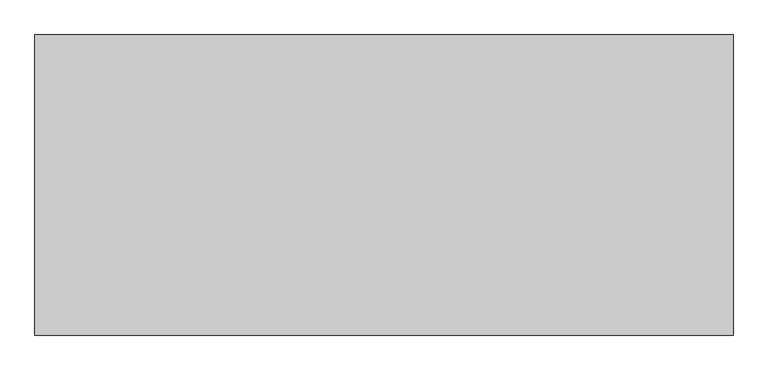
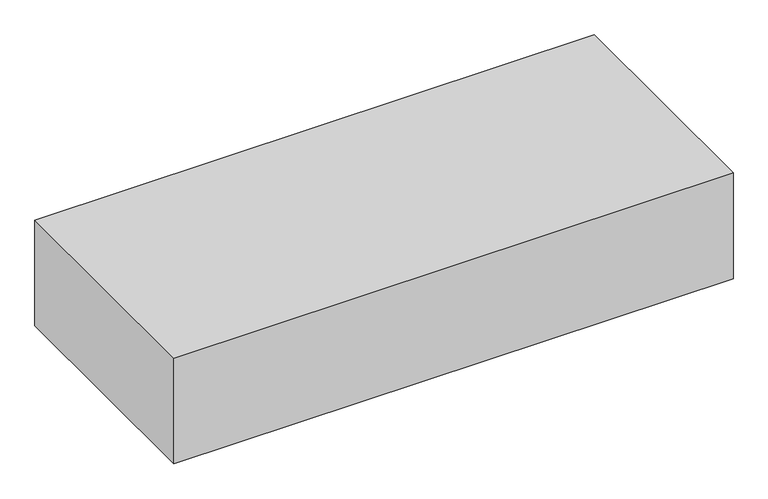
"""IFC4 building model written with IfcOpenShell, lengths in millimetres: proxy geometry."""

from ifc_helpers import new_model, si_unit, origin, place, context, project, spatial, faceted_brep, source, transform, mapped, element, save


def generic_models_374839be(model_context):
    return source(origin(), model_context, "Body", "Brep", [
        faceted_brep([(-1233.1005972, -1591.9129108, 304.8), (290.8994028, -1591.9129108, 304.8), (290.8994028, -936.8072249, 304.8), (-1233.1005972, -936.8072249, 304.8), (-1233.1005972, -1591.9129108, 0.0), (-1233.1005972, -936.8072249, 0.0), (290.8994028, -936.8072249, 0.0), (290.8994028, -1591.9129108, 0.0), (-1182.3005972, -936.8072249, 254.0), (-1182.3005972, -936.8072249, 75.4468045), (240.0994028, -936.8072249, 75.4468045), (240.0994028, -936.8072249, 254.0), (-1182.3005972, -1546.4072249, 254.0), (240.0994028, -1546.4072249, 254.0), (240.0994028, -1546.4072249, 75.4468045), (-1182.3005972, -1546.4072249, 75.4468045)], [[[0, 1, 2, 3]], [[4, 5, 6, 7]], [[1, 0, 4, 7]], [[2, 1, 7, 6]], [[3, 2, 6, 5], [8, 9, 10, 11]], [[0, 3, 5, 4]], [[12, 13, 14, 15]], [[12, 15, 9, 8]], [[15, 14, 10, 9]], [[14, 13, 11, 10]], [[13, 12, 8, 11]]]),
    ])


if __name__ == "__main__":
    model = new_model("IFC4")
    model_context = context("Model", 3, world=origin())
    ifc_project = project(units=[si_unit("LENGTHUNIT", "METRE", prefix="MILLI")], contexts=[model_context])
    site = spatial("IfcSite", under=ifc_project)
    building = spatial("IfcBuilding", under=site)
    placement = place(None, origin())
    generic_models_shape = generic_models_374839be(model_context)
    element("IfcBuildingElementProxy", 1, Name="Generic Models", at=placement, inside=building, context=model_context, shape_type="MappedRepresentation", body=[
        mapped(generic_models_shape, transform((0.0, 0.0, 0.0), x_axis=(1.0, 0.0, 0.0), y_axis=(0.0, 1.0, 0.0), z_axis=(0.0, 0.0, 1.0))),
    ])
    save(model, "model.ifc")

# Revit data of these elements
# Element 1 (IfcBuildingElementProxy)
#   Materials on its faces: "Door - Panel"
# Materials
#   "Door - Panel": class "Wood", colour RGB 210 159 95, transparency 0, Cost = 0
